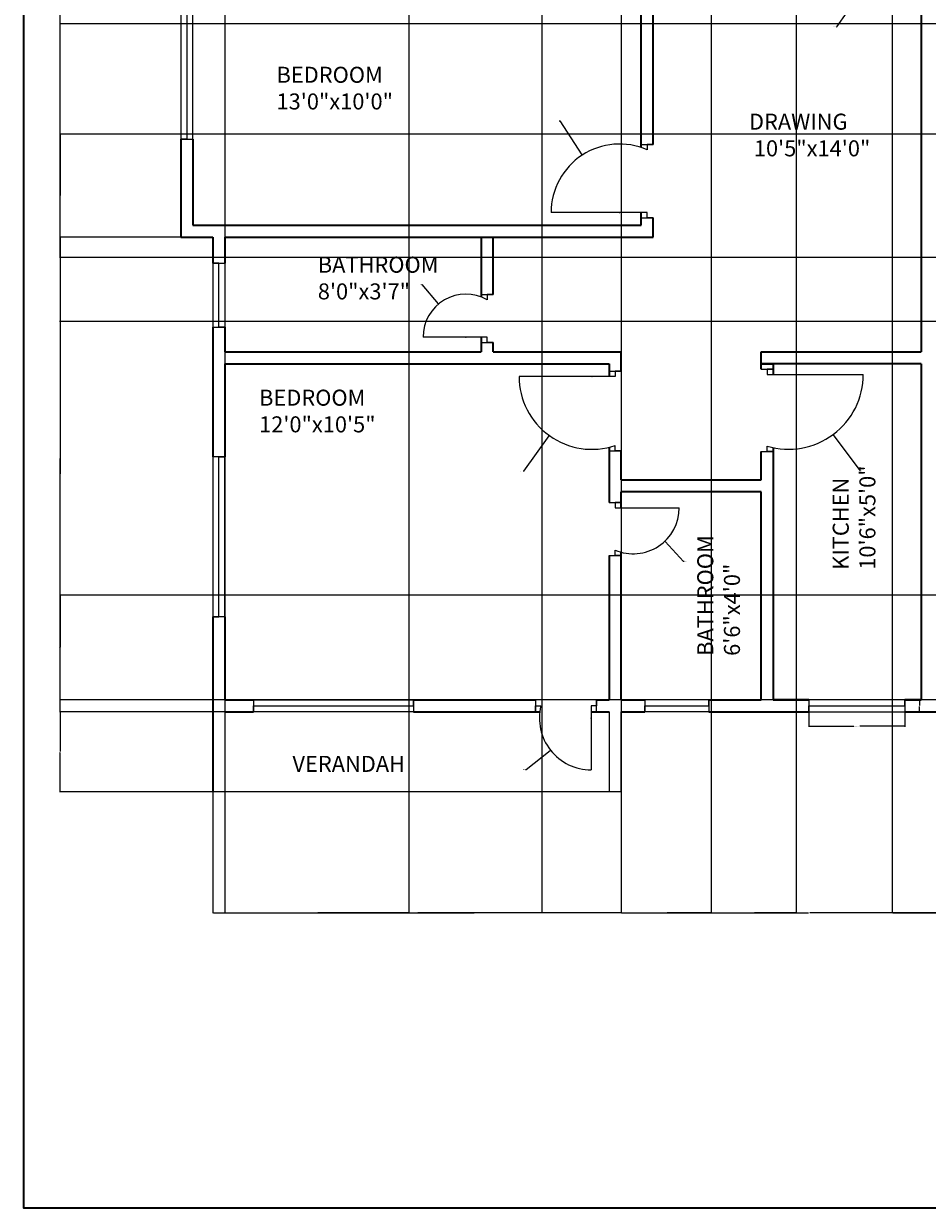
# Model space of a CAD drawing. Units: inches. Extents: x 1831 to 2867, y 1605 to 2524.
# Tile 1 of 7: x 1831 to 2170, y 1605 to 2049. Entities that reach past the tile are written whole.
import ezdxf

# ---------------------------------------------------------------- set-up
doc = ezdxf.new("R2010")
doc.units = ezdxf.units.IN
for name, color, linetype, lineweight in [('A-ANNO-DIMS', 2, 'Continuous', 18), ('A-ANNO-TTLB', 7, 'Continuous', 35), ('A-AREA-IDEN', 7, 'Continuous', 18), ('A-DOOR', 11, 'Continuous', 18), ('A-FLOR-BALC', 7, 'Continuous', 25), ('A-GLAZ', 121, 'Continuous', 18), ('A-WALL', 7, 'Continuous', 35)]:
    doc.layers.add(name, color=color, linetype=linetype, lineweight=lineweight)
doc.styles.get("Standard").update_dxf_attribs({"font": 'arial.ttf'})
doc.dimstyles.get("Standard").update_dxf_attribs({"dimtxt": 0.18, "dimasz": 0.18, "dimexe": 0.18, "dimexo": 0.0625, "dimgap": 0.09, "dimtad": 0, "dimtih": 1, "dimtoh": 1, "dimdec": 4, "dimzin": 0, "dimdsep": 46, "dimtxsty": 'Standard', "dimcen": 0.09, "dimadec": 0, "dimazin": 0, "dimtfac": 1, "dimtdec": 4, "dimtofl": 0, "dimtmove": 0, "dimatfit": 3, "dimfxl": 1, "dimtolj": 1, "dimtzin": 0, "dimarcsym": 0})

# ---------------------------------------------------------------- blocks, each defined once
blk = doc.blocks.new('WIN-60IN')
for p, q in [((4.5, 60), (0, 60)), ((0, 60), (2.25, 60)), ((0, 0), (0, 60)), ((2.25, 60), (2.25, 0)), ((4.5, 60), (4.5, 0)), ((4.5, 0), (0, 0)), ((2.25, 0), (4.5, 0))]:
    blk.add_line(p, q)
blk = doc.blocks.new('WIN-24IN')
for p, q in [((4.5, 24), (0, 24)), ((0, 24), (2.25, 24)), ((0, 0), (0, 24)), ((2.25, 24), (2.25, 0)), ((4.5, 0), (4.5, 24)), ((4.5, 0), (0, 0)), ((2.25, 0), (4.5, 0))]:
    blk.add_line(p, q)
blk = doc.blocks.new('WIN-36IN')
for p, q in [((0, 0), (0, 4.5)), ((36, 4.5), (0, 4.5)), ((36, 0), (36, 4.5)), ((36, 4.5), (36, 2.25)), ((36, 2.25), (0, 2.25)), ((0, 2.25), (0, 0)), ((0, 0), (36, 0))]:
    blk.add_line(p, q)
blk = doc.blocks.new('DOOR-LEAF-36IN')
for p, q in [((0, 2), (4.5, 2)), ((4.5, 2), (2.25, 2)), ((2.25, 2), (2.25, 0)), ((2.25, 0), (38.25, 0))]:
    blk.add_line(p, q)
blk = doc.blocks.new('DOOR-LEAF-36IN-ALT')
for p, q in [((36, 2), (0, 2)), ((33.75, 0), (38.25, 0)), ((36, 0), (36, 2)), ((38.25, 0), (36, 0))]:
    blk.add_line(p, q)
blk = doc.blocks.new('DOOR-LEAF-24IN')
for p, q in [((2.25, 0), (2.25, 2)), ((2.25, 2), (26.25, 2)), ((0, 0), (4.5, 0)), ((4.5, 0), (2.25, 0))]:
    blk.add_line(p, q)
blk = doc.blocks.new('DOOR-LEAF-24IN-ALT')
for p, q in [((24, 2), (0, 2)), ((21.75, 0), (26.25, 0)), ((24, 0), (24, 2)), ((26.25, 0), (24, 0))]:
    blk.add_line(p, q)
blk = doc.blocks.new('DOOR-STRIKE-JAMB')
for p, q in [((0, 0), (4.5, 0)), ((2.25, 0), (2.25, 2)), ((4.5, 0), (2.25, 0))]:
    blk.add_line(p, q)
blk = doc.blocks.new('*D18')
at = {"layer": 'A-ANNO-DIMS', "color": 0, "lineweight": -2, "transparency": 16777216}
for p, q in [((2125.43, 1791.11), (2125.43, 1785.59)), ((2161.43, 1791.11), (2161.43, 1785.59)), ((2125.61, 1785.77), (2142.31, 1785.77)), ((2161.25, 1785.77), (2144.55, 1785.77))]:
    blk.add_line(p, q, dxfattribs=at)
at = {"layer": 'A-ANNO-DIMS', "color": 0, "transparency": 16777216}
for points in [[(2125.61, 1785.8), (2125.61, 1785.74), (2125.43, 1785.77)], [(2161.25, 1785.8), (2161.25, 1785.74), (2161.43, 1785.77)]]:
    blk.add_solid(points, dxfattribs=at)
at = {"layer": 'Defpoints', "color": 0, "transparency": 16777216}
for p in [(2125.43, 1791.17), (2161.43, 1791.17), (2125.43, 1785.77)]:
    blk.add_point(p, dxfattribs=at)
at = {"layer": 'A-ANNO-DIMS', "color": 0, "transparency": 16777216, "insert": (2143.43, 1785.77), "char_height": 0.18, "attachment_point": 5}
blk.add_mtext('\\A1;WINDOW 36 TYP.', dxfattribs=at)
blk = doc.blocks.new('*D19')
at = {"layer": 'A-ANNO-DIMS', "color": 0, "lineweight": -2, "transparency": 16777216}
for p, q in [((2161.49, 1795.67), (2167.01, 1795.67)), ((2166.83, 1795.49), (2166.83, 1793.61)), ((2161.49, 1791.17), (2167.01, 1791.17)), ((2166.83, 1791.35), (2166.83, 1793.24))]:
    blk.add_line(p, q, dxfattribs=at)
at = {"layer": 'A-ANNO-DIMS', "color": 0, "transparency": 16777216}
for points in [[(2166.8, 1795.49), (2166.86, 1795.49), (2166.83, 1795.67)], [(2166.8, 1791.35), (2166.86, 1791.35), (2166.83, 1791.17)]]:
    blk.add_solid(points, dxfattribs=at)
at = {"layer": 'Defpoints', "color": 0, "transparency": 16777216}
for p in [(2161.43, 1795.67), (2161.43, 1791.17), (2166.83, 1791.17)]:
    blk.add_point(p, dxfattribs=at)
at = {"layer": 'A-ANNO-DIMS', "color": 0, "transparency": 16777216, "insert": (2166.83, 1793.42), "char_height": 0.18, "attachment_point": 5}
blk.add_mtext('\\A1;5 TYP.', dxfattribs=at)
blk = doc.blocks.new('*D24')
at = {"layer": 'A-ANNO-DIMS', "color": 0, "lineweight": -2, "transparency": 16777216}
for p, q in [((1902.05, 1761.11), (1902.05, 1715.69)), ((2055.05, 1761.11), (2055.05, 1715.69)), ((1902.23, 1715.87), (1978.27, 1715.87)), ((2054.87, 1715.87), (1978.83, 1715.87))]:
    blk.add_line(p, q, dxfattribs=at)
at = {"layer": 'A-ANNO-DIMS', "color": 0, "transparency": 16777216}
for points in [[(1902.23, 1715.9), (1902.23, 1715.84), (1902.05, 1715.87)], [(2054.87, 1715.9), (2054.87, 1715.84), (2055.05, 1715.87)]]:
    blk.add_solid(points, dxfattribs=at)
at = {"layer": 'Defpoints', "color": 0, "transparency": 16777216}
for p in [(1902.05, 1761.17), (2055.05, 1761.17), (2055.05, 1715.87)]:
    blk.add_point(p, dxfattribs=at)
at = {"layer": 'A-ANNO-DIMS', "color": 0, "transparency": 16777216, "insert": (1978.55, 1715.87), "char_height": 0.18, "attachment_point": 5}
blk.add_mtext('\\A1;153', dxfattribs=at)
blk = doc.blocks.new('*D25')
at = {"layer": 'A-ANNO-DIMS', "color": 0, "lineweight": -2, "transparency": 16777216}
for p, q in [((2055.05, 1761.11), (2055.05, 1715.69)), ((2196.05, 1761.11), (2196.05, 1715.69)), ((2055.23, 1715.87), (2125.29, 1715.87)), ((2195.87, 1715.87), (2125.81, 1715.87))]:
    blk.add_line(p, q, dxfattribs=at)
at = {"layer": 'A-ANNO-DIMS', "color": 0, "transparency": 16777216}
for points in [[(2055.23, 1715.9), (2055.23, 1715.84), (2055.05, 1715.87)], [(2195.87, 1715.9), (2195.87, 1715.84), (2196.05, 1715.87)]]:
    blk.add_solid(points, dxfattribs=at)
at = {"layer": 'Defpoints', "color": 0, "transparency": 16777216}
for p in [(2055.05, 1761.17), (2196.05, 1761.17), (2196.05, 1715.87)]:
    blk.add_point(p, dxfattribs=at)
at = {"layer": 'A-ANNO-DIMS', "color": 0, "transparency": 16777216, "insert": (2125.55, 1715.87), "char_height": 0.18, "attachment_point": 5}
blk.add_mtext('\\A1;141', dxfattribs=at)
blk = doc.blocks.new('*D33')
at = {"layer": 'A-ANNO-DIMS', "color": 0, "lineweight": -2, "transparency": 16777216}
for p, q in [((1889.99, 2218.17), (1844.57, 2218.17)), ((1844.75, 2217.99), (1844.75, 2093.86)), ((1844.75, 1969.35), (1844.75, 2093.49)), ((1889.99, 1969.17), (1844.57, 1969.17))]:
    blk.add_line(p, q, dxfattribs=at)
at = {"layer": 'A-ANNO-DIMS', "color": 0, "transparency": 16777216}
for points in [[(1844.72, 2217.99), (1844.78, 2217.99), (1844.75, 2218.17)], [(1844.72, 1969.35), (1844.78, 1969.35), (1844.75, 1969.17)]]:
    blk.add_solid(points, dxfattribs=at)
at = {"layer": 'Defpoints', "color": 0, "transparency": 16777216}
for p in [(1890.05, 2218.17), (1844.75, 1969.17), (1890.05, 1969.17)]:
    blk.add_point(p, dxfattribs=at)
at = {"layer": 'A-ANNO-DIMS', "color": 0, "transparency": 16777216, "insert": (1844.75, 2093.67), "char_height": 0.18, "attachment_point": 5}
blk.add_mtext('\\A1;249', dxfattribs=at)
blk = doc.blocks.new('*D34')
at = {"layer": 'A-ANNO-DIMS', "color": 0, "lineweight": -2, "transparency": 16777216}
for p, q in [((1901.99, 1969.17), (1844.57, 1969.17)), ((1844.75, 1968.99), (1844.75, 1880.36)), ((1844.75, 1791.35), (1844.75, 1879.99)), ((1906.49, 1791.17), (1844.57, 1791.17))]:
    blk.add_line(p, q, dxfattribs=at)
at = {"layer": 'A-ANNO-DIMS', "color": 0, "transparency": 16777216}
for points in [[(1844.72, 1968.99), (1844.78, 1968.99), (1844.75, 1969.17)], [(1844.72, 1791.35), (1844.78, 1791.35), (1844.75, 1791.17)]]:
    blk.add_solid(points, dxfattribs=at)
at = {"layer": 'Defpoints', "color": 0, "transparency": 16777216}
for p in [(1902.05, 1969.17), (1844.75, 1791.17), (1906.55, 1791.17)]:
    blk.add_point(p, dxfattribs=at)
at = {"layer": 'A-ANNO-DIMS', "color": 0, "transparency": 16777216, "insert": (1844.75, 1880.17), "char_height": 0.18, "attachment_point": 5}
blk.add_mtext('\\A1;178', dxfattribs=at)
blk = doc.blocks.new('*D35')
at = {"layer": 'A-ANNO-DIMS', "color": 0, "lineweight": -2, "transparency": 16777216}
for p, q in [((1906.49, 1791.17), (1844.57, 1791.17)), ((1844.75, 1790.99), (1844.75, 1776.36)), ((1844.75, 1761.35), (1844.75, 1775.99)), ((1901.99, 1761.17), (1844.57, 1761.17))]:
    blk.add_line(p, q, dxfattribs=at)
at = {"layer": 'A-ANNO-DIMS', "color": 0, "transparency": 16777216}
for points in [[(1844.72, 1790.99), (1844.78, 1790.99), (1844.75, 1791.17)], [(1844.72, 1761.35), (1844.78, 1761.35), (1844.75, 1761.17)]]:
    blk.add_solid(points, dxfattribs=at)
at = {"layer": 'Defpoints', "color": 0, "transparency": 16777216}
for p in [(1906.55, 1791.17), (1844.75, 1761.17), (1902.05, 1761.17)]:
    blk.add_point(p, dxfattribs=at)
at = {"layer": 'A-ANNO-DIMS', "color": 0, "transparency": 16777216, "insert": (1844.75, 1776.17), "char_height": 0.18, "attachment_point": 5}
blk.add_mtext('\\A1;30', dxfattribs=at)
blk = doc.blocks.new('*D37')
at = {"layer": 'A-ANNO-DIMS', "color": 0, "lineweight": -2, "transparency": 16777216}
for p, q in [((1906.55, 2387.11), (1906.55, 1715.69)), ((1975.47, 2387.11), (1975.47, 1715.69)), ((1906.73, 1715.87), (1940.62, 1715.87)), ((1975.29, 1715.87), (1941.4, 1715.87))]:
    blk.add_line(p, q, dxfattribs=at)
at = {"layer": 'A-ANNO-DIMS', "color": 0, "transparency": 16777216}
for points in [[(1906.73, 1715.9), (1906.73, 1715.84), (1906.55, 1715.87)], [(1975.29, 1715.9), (1975.29, 1715.84), (1975.47, 1715.87)]]:
    blk.add_solid(points, dxfattribs=at)
at = {"layer": 'Defpoints', "color": 0, "transparency": 16777216}
for p in [(1906.55, 2387.17), (1975.47, 2387.17), (1975.47, 1715.87)]:
    blk.add_point(p, dxfattribs=at)
at = {"layer": 'A-ANNO-DIMS', "color": 0, "transparency": 16777216, "insert": (1941.01, 1715.87), "char_height": 0.18, "attachment_point": 5}
blk.add_mtext('\\A1;68.92', dxfattribs=at)
blk = doc.blocks.new('*D38')
at = {"layer": 'A-ANNO-DIMS', "color": 0, "lineweight": -2, "transparency": 16777216}
for p, q in [((1975.47, 2391.61), (1975.47, 1715.69)), ((2025.28, 2391.61), (2025.28, 1715.69)), ((1975.65, 1715.87), (1999.99, 1715.87)), ((2025.1, 1715.87), (2000.75, 1715.87))]:
    blk.add_line(p, q, dxfattribs=at)
at = {"layer": 'A-ANNO-DIMS', "color": 0, "transparency": 16777216}
for points in [[(1975.65, 1715.9), (1975.65, 1715.84), (1975.47, 1715.87)], [(2025.1, 1715.9), (2025.1, 1715.84), (2025.28, 1715.87)]]:
    blk.add_solid(points, dxfattribs=at)
at = {"layer": 'Defpoints', "color": 0, "transparency": 16777216}
for p in [(1975.47, 2391.67), (2025.28, 2391.67), (2025.28, 1715.87)]:
    blk.add_point(p, dxfattribs=at)
at = {"layer": 'A-ANNO-DIMS', "color": 0, "transparency": 16777216, "insert": (2000.37, 1715.87), "char_height": 0.18, "attachment_point": 5}
blk.add_mtext('\\A1;49.81', dxfattribs=at)
blk = doc.blocks.new('*D39')
at = {"layer": 'A-ANNO-DIMS', "color": 0, "lineweight": -2, "transparency": 16777216}
for p, q in [((2055.05, 2387.11), (2055.05, 1715.69)), ((2088.73, 2387.11), (2088.73, 1715.69)), ((2055.23, 1715.87), (2071.5, 1715.87)), ((2088.55, 1715.87), (2072.28, 1715.87))]:
    blk.add_line(p, q, dxfattribs=at)
at = {"layer": 'A-ANNO-DIMS', "color": 0, "transparency": 16777216}
for points in [[(2055.23, 1715.9), (2055.23, 1715.84), (2055.05, 1715.87)], [(2088.55, 1715.9), (2088.55, 1715.84), (2088.73, 1715.87)]]:
    blk.add_solid(points, dxfattribs=at)
at = {"layer": 'Defpoints', "color": 0, "transparency": 16777216}
for p in [(2055.05, 2387.17), (2088.73, 2387.17), (2088.73, 1715.87)]:
    blk.add_point(p, dxfattribs=at)
at = {"layer": 'A-ANNO-DIMS', "color": 0, "transparency": 16777216, "insert": (2071.89, 1715.87), "char_height": 0.18, "attachment_point": 5}
blk.add_mtext('\\A1;33.68', dxfattribs=at)
blk = doc.blocks.new('*D40')
at = {"layer": 'A-ANNO-DIMS', "color": 0, "lineweight": -2, "transparency": 16777216}
for p, q in [((2088.73, 2387.11), (2088.73, 1715.69)), ((2120.64, 2387.11), (2120.64, 1715.69)), ((2088.91, 1715.87), (2104.31, 1715.87)), ((2120.46, 1715.87), (2105.06, 1715.87))]:
    blk.add_line(p, q, dxfattribs=at)
at = {"layer": 'A-ANNO-DIMS', "color": 0, "transparency": 16777216}
for points in [[(2088.91, 1715.9), (2088.91, 1715.84), (2088.73, 1715.87)], [(2120.46, 1715.9), (2120.46, 1715.84), (2120.64, 1715.87)]]:
    blk.add_solid(points, dxfattribs=at)
at = {"layer": 'Defpoints', "color": 0, "transparency": 16777216}
for p in [(2088.73, 2387.17), (2120.64, 2387.17), (2120.64, 1715.87)]:
    blk.add_point(p, dxfattribs=at)
at = {"layer": 'A-ANNO-DIMS', "color": 0, "transparency": 16777216, "insert": (2104.69, 1715.87), "char_height": 0.18, "attachment_point": 5}
blk.add_mtext('\\A1;31.91', dxfattribs=at)
blk = doc.blocks.new('*D41')
at = {"layer": 'A-ANNO-DIMS', "color": 0, "lineweight": -2, "transparency": 16777216}
for p, q in [((2156.64, 2387.11), (2156.64, 1715.69)), ((2210.17, 2387.11), (2210.17, 1715.69)), ((2156.82, 1715.87), (2183.01, 1715.87)), ((2209.99, 1715.87), (2183.8, 1715.87))]:
    blk.add_line(p, q, dxfattribs=at)
at = {"layer": 'A-ANNO-DIMS', "color": 0, "transparency": 16777216}
for points in [[(2156.82, 1715.9), (2156.82, 1715.84), (2156.64, 1715.87)], [(2209.99, 1715.9), (2209.99, 1715.84), (2210.17, 1715.87)]]:
    blk.add_solid(points, dxfattribs=at)
at = {"layer": 'Defpoints', "color": 0, "transparency": 16777216}
for p in [(2156.64, 2387.17), (2210.17, 2387.17), (2210.17, 1715.87)]:
    blk.add_point(p, dxfattribs=at)
at = {"layer": 'A-ANNO-DIMS', "color": 0, "transparency": 16777216, "insert": (2183.4, 1715.87), "char_height": 0.18, "attachment_point": 5}
blk.add_mtext('\\A1;53.52', dxfattribs=at)
blk = doc.blocks.new('*D53')
at = {"layer": 'A-ANNO-DIMS', "color": 0, "lineweight": -2, "transparency": 16777216}
for p, q in [((2786.99, 2007.7), (1844.57, 2007.7)), ((1844.75, 2007.52), (1844.75, 1984.78)), ((1844.75, 1961.67), (1844.75, 1984.41)), ((2786.99, 1961.49), (1844.57, 1961.49))]:
    blk.add_line(p, q, dxfattribs=at)
at = {"layer": 'A-ANNO-DIMS', "color": 0, "transparency": 16777216}
for points in [[(1844.72, 2007.52), (1844.78, 2007.52), (1844.75, 2007.7)], [(1844.72, 1961.67), (1844.78, 1961.67), (1844.75, 1961.49)]]:
    blk.add_solid(points, dxfattribs=at)
at = {"layer": 'Defpoints', "color": 0, "transparency": 16777216}
for p in [(2787.05, 2007.7), (1844.75, 1961.49), (2787.05, 1961.49)]:
    blk.add_point(p, dxfattribs=at)
at = {"layer": 'A-ANNO-DIMS', "color": 0, "transparency": 16777216, "insert": (1844.75, 1984.59), "char_height": 0.18, "attachment_point": 5}
blk.add_mtext('\\A1;46.2', dxfattribs=at)
blk = doc.blocks.new('*D54')
at = {"layer": 'A-ANNO-DIMS', "color": 0, "lineweight": -2, "transparency": 16777216}
for p, q in [((2786.99, 1937.49), (1844.57, 1937.49)), ((1844.75, 1937.31), (1844.75, 1886.37)), ((1844.75, 1835.06), (1844.75, 1886)), ((2786.99, 1834.88), (1844.57, 1834.88))]:
    blk.add_line(p, q, dxfattribs=at)
at = {"layer": 'A-ANNO-DIMS', "color": 0, "transparency": 16777216}
for points in [[(1844.72, 1937.31), (1844.78, 1937.31), (1844.75, 1937.49)], [(1844.72, 1835.06), (1844.78, 1835.06), (1844.75, 1834.88)]]:
    blk.add_solid(points, dxfattribs=at)
at = {"layer": 'Defpoints', "color": 0, "transparency": 16777216}
for p in [(2787.05, 1937.49), (1844.75, 1834.88), (2787.05, 1834.88)]:
    blk.add_point(p, dxfattribs=at)
at = {"layer": 'A-ANNO-DIMS', "color": 0, "transparency": 16777216, "insert": (1844.75, 1886.19), "char_height": 0.18, "attachment_point": 5}
blk.add_mtext('\\A1;102.61', dxfattribs=at)
blk = doc.blocks.new('*D55')
at = {"layer": 'A-ANNO-DIMS', "color": 0, "lineweight": -2, "transparency": 16777216}
for p, q in [((2786.99, 1834.88), (1844.57, 1834.88)), ((1844.75, 1834.7), (1844.75, 1815.46)), ((1844.75, 1795.85), (1844.75, 1815.09)), ((2786.99, 1795.67), (1844.57, 1795.67))]:
    blk.add_line(p, q, dxfattribs=at)
at = {"layer": 'A-ANNO-DIMS', "color": 0, "transparency": 16777216}
for points in [[(1844.72, 1834.7), (1844.78, 1834.7), (1844.75, 1834.88)], [(1844.72, 1795.85), (1844.78, 1795.85), (1844.75, 1795.67)]]:
    blk.add_solid(points, dxfattribs=at)
at = {"layer": 'Defpoints', "color": 0, "transparency": 16777216}
for p in [(2787.05, 1834.88), (1844.75, 1795.67), (2787.05, 1795.67)]:
    blk.add_point(p, dxfattribs=at)
at = {"layer": 'A-ANNO-DIMS', "color": 0, "transparency": 16777216, "insert": (1844.75, 1815.28), "char_height": 0.18, "attachment_point": 5}
blk.add_mtext('\\A1;39.206', dxfattribs=at)
blk = doc.blocks.new('*D60')
at = {"layer": 'A-ANNO-DIMS', "color": 0, "lineweight": -2, "transparency": 16777216}
for p, q in [((2225.43, 2091.42), (1844.57, 2091.42)), ((1844.75, 2091.24), (1844.75, 2070.48)), ((1844.75, 2049.35), (1844.75, 2070.12)), ((2225.43, 2049.17), (1844.57, 2049.17))]:
    blk.add_line(p, q, dxfattribs=at)
at = {"layer": 'A-ANNO-DIMS', "color": 0, "transparency": 16777216}
for points in [[(1844.72, 2091.24), (1844.78, 2091.24), (1844.75, 2091.42)], [(1844.72, 2049.35), (1844.78, 2049.35), (1844.75, 2049.17)]]:
    blk.add_solid(points, dxfattribs=at)
at = {"layer": 'Defpoints', "color": 0, "transparency": 16777216}
for p in [(1844.75, 2091.42), (2225.49, 2091.42), (2225.49, 2049.17)]:
    blk.add_point(p, dxfattribs=at)
at = {"layer": 'A-ANNO-DIMS', "color": 0, "transparency": 16777216, "insert": (1844.75, 2070.3), "char_height": 0.18, "attachment_point": 5}
blk.add_mtext('\\A1;42.25', dxfattribs=at)
blk = doc.blocks.new('*D73')
at = {"layer": 'A-ANNO-DIMS', "color": 0, "lineweight": -2, "transparency": 16777216}
for p, q in [((2117.68, 1917.66), (2117.86, 1917.66)), ((2117.77, 1917.57), (2117.77, 1917.75)), ((2144.6, 1881.73), (2134.65, 1895.06)), ((2144.78, 1881.73), (2144.6, 1881.73))]:
    blk.add_line(p, q, dxfattribs=at)
at = {"layer": 'A-ANNO-DIMS', "color": 0, "transparency": 16777216}
blk.add_solid([(2134.67, 1895.08), (2134.62, 1895.04), (2134.54, 1895.2)], dxfattribs=at)
at = {"layer": 'Defpoints', "color": 0, "transparency": 16777216}
for p in [(2117.77, 1917.66), (2134.54, 1895.2)]:
    blk.add_point(p, dxfattribs=at)
at = {"layer": 'A-ANNO-DIMS', "color": 0, "transparency": 16777216, "insert": (2145.26, 1881.73), "char_height": 0.18, "attachment_point": 5}
blk.add_mtext('\\A1;R28.03', dxfattribs=at)
blk = doc.blocks.new('*D77')
at = {"layer": 'A-ANNO-DIMS', "color": 0, "lineweight": -2, "transparency": 16777216}
for p, q in [((2044.03, 1916.93), (2044.21, 1916.93)), ((2044.12, 1916.84), (2044.12, 1917.02)), ((2018.59, 1881.45), (2028.06, 1894.61)), ((2018.41, 1881.45), (2018.59, 1881.45))]:
    blk.add_line(p, q, dxfattribs=at)
at = {"layer": 'A-ANNO-DIMS', "color": 0, "transparency": 16777216}
blk.add_solid([(2028.04, 1894.63), (2028.08, 1894.59), (2028.17, 1894.76)], dxfattribs=at)
at = {"layer": 'Defpoints', "color": 0, "transparency": 16777216}
for p in [(2044.12, 1916.93), (2028.17, 1894.76)]:
    blk.add_point(p, dxfattribs=at)
at = {"layer": 'A-ANNO-DIMS', "color": 0, "transparency": 16777216, "insert": (2017.86, 1881.45), "char_height": 0.18, "attachment_point": 5}
blk.add_mtext('\\A1;R27.315', dxfattribs=at)
blk = doc.blocks.new('*D79')
at = {"layer": 'A-ANNO-DIMS', "color": 0, "lineweight": -2, "transparency": 16777216}
for p, q in [((2160.66, 2083.26), (2160.84, 2083.26)), ((2160.75, 2083.17), (2160.75, 2083.35)), ((2135.91, 2048.03), (2145.12, 2061.09)), ((2135.73, 2048.03), (2135.91, 2048.03))]:
    blk.add_line(p, q, dxfattribs=at)
at = {"layer": 'A-ANNO-DIMS', "color": 0, "transparency": 16777216}
blk.add_solid([(2145.09, 2061.11), (2145.14, 2061.08), (2145.22, 2061.24)], dxfattribs=at)
at = {"layer": 'Defpoints', "color": 0, "transparency": 16777216}
for p in [(2160.75, 2083.26), (2145.22, 2061.24)]:
    blk.add_point(p, dxfattribs=at)
at = {"layer": 'A-ANNO-DIMS', "color": 0, "transparency": 16777216, "insert": (2135.18, 2048.03), "char_height": 0.18, "attachment_point": 5}
blk.add_mtext('\\A1;R26.945', dxfattribs=at)
blk = doc.blocks.new('*D83')
at = {"layer": 'A-ANNO-DIMS', "color": 0, "lineweight": -2, "transparency": 16777216}
for p, q in [((2031.86, 2012.78), (2032.04, 2012.78)), ((2032.04, 2012.78), (2040.34, 2000.04)), ((2054.36, 1978.4), (2054.54, 1978.4)), ((2054.45, 1978.31), (2054.45, 1978.49))]:
    blk.add_line(p, q, dxfattribs=at)
at = {"layer": 'A-ANNO-DIMS', "color": 0, "transparency": 16777216}
blk.add_solid([(2040.37, 2000.05), (2040.32, 2000.02), (2040.44, 1999.89)], dxfattribs=at)
at = {"layer": 'Defpoints', "color": 0, "transparency": 16777216}
for p in [(2040.44, 1999.89), (2054.45, 1978.4)]:
    blk.add_point(p, dxfattribs=at)
at = {"layer": 'A-ANNO-DIMS', "color": 0, "transparency": 16777216, "insert": (2031.38, 2012.78), "char_height": 0.18, "attachment_point": 5}
blk.add_mtext('\\A1;R25.65', dxfattribs=at)
blk = doc.blocks.new('*D87')
at = {"layer": 'A-ANNO-DIMS', "color": 0, "lineweight": -2, "transparency": 16777216}
for p, q in [((2043.75, 1788.85), (2043.93, 1788.85)), ((2043.84, 1788.76), (2043.84, 1788.94)), ((2019.41, 1769.63), (2028.43, 1776.73)), ((2019.23, 1769.63), (2019.41, 1769.63))]:
    blk.add_line(p, q, dxfattribs=at)
at = {"layer": 'A-ANNO-DIMS', "color": 0, "transparency": 16777216}
blk.add_solid([(2028.41, 1776.75), (2028.45, 1776.7), (2028.57, 1776.84)], dxfattribs=at)
at = {"layer": 'Defpoints', "color": 0, "transparency": 16777216}
for p in [(2043.84, 1788.85), (2028.57, 1776.84)]:
    blk.add_point(p, dxfattribs=at)
at = {"layer": 'A-ANNO-DIMS', "color": 0, "transparency": 16777216, "insert": (2018.68, 1769.63), "char_height": 0.18, "attachment_point": 5}
blk.add_mtext('\\A1;R19.428', dxfattribs=at)
blk = doc.blocks.new('*D96')
at = {"layer": 'A-ANNO-DIMS', "color": 0, "lineweight": -2, "transparency": 16777216}
for p, q in [((1980.19, 1951.42), (1980.37, 1951.42)), ((1980.37, 1951.42), (1986.44, 1944.17)), ((1996.77, 1931.71), (1996.95, 1931.71)), ((1996.86, 1931.62), (1996.86, 1931.8))]:
    blk.add_line(p, q, dxfattribs=at)
at = {"layer": 'A-ANNO-DIMS', "color": 0, "transparency": 16777216}
blk.add_solid([(1986.46, 1944.19), (1986.42, 1944.15), (1986.56, 1944.03)], dxfattribs=at)
at = {"layer": 'Defpoints', "color": 0, "transparency": 16777216}
for p in [(1986.56, 1944.03), (1996.86, 1931.71)]:
    blk.add_point(p, dxfattribs=at)
at = {"layer": 'A-ANNO-DIMS', "color": 0, "transparency": 16777216, "insert": (1979.71, 1951.42), "char_height": 0.18, "attachment_point": 5}
blk.add_mtext('\\A1;R16.06', dxfattribs=at)
blk = doc.blocks.new('*D97')
at = {"layer": 'A-ANNO-DIMS', "color": 0, "lineweight": -2, "transparency": 16777216}
for p, q in [((2059.48, 1867.69), (2059.66, 1867.69)), ((2059.57, 1867.6), (2059.57, 1867.78)), ((2078.45, 1847.6), (2071.5, 1855)), ((2078.63, 1847.6), (2078.45, 1847.6))]:
    blk.add_line(p, q, dxfattribs=at)
at = {"layer": 'A-ANNO-DIMS', "color": 0, "transparency": 16777216}
blk.add_solid([(2071.52, 1855.02), (2071.47, 1854.98), (2071.37, 1855.14)], dxfattribs=at)
at = {"layer": 'Defpoints', "color": 0, "transparency": 16777216}
for p in [(2059.57, 1867.69), (2071.37, 1855.14)]:
    blk.add_point(p, dxfattribs=at)
at = {"layer": 'A-ANNO-DIMS', "color": 0, "transparency": 16777216, "insert": (2079.11, 1847.6), "char_height": 0.18, "attachment_point": 5}
blk.add_mtext('\\A1;R17.23', dxfattribs=at)

msp = doc.modelspace()

# ---------------------------------------------------------------- linework, layer by layer
at = {"layer": 'A-ANNO-TTLB'}
msp.add_lwpolyline([(1831.1248, 2523.9204), (2867.0416, 2523.9204), (2867.0416, 1605.0781), (1831.1248, 1605.0781)], close=True, dxfattribs=at)
at = {"layer": 'A-DOOR'}
for centre, radius, start, end in [((2054.453, 1978.3983), 25.6519, 66.208959, 180), ((1996.8625, 1931.7112), 16.0615, 60.379406, 180), ((2044.1157, 1916.9308), 27.3147, 180, 288.540393), ((2117.7728, 1917.6648), 28.0282, 253.475877, 360), ((2059.5721, 1867.688), 17.2289, 246.858029, 360), ((2043.8406, 1788.8513), 19.4276, 166.38723, 270)]:
    msp.add_arc(centre, radius, start, end, dxfattribs=at)
at = {"layer": 'A-FLOR-BALC'}
for p, q in [((1906.551, 1791.1738), (1906.551, 1761.1738)), ((2050.551, 1791.1738), (2050.551, 1761.1738)), ((2055.051, 1761.1738), (2055.051, 1791.1738)), ((2055.051, 1761.1738), (1902.051, 1761.1738))]:
    msp.add_line(p, q, dxfattribs=at)
at = {"layer": 'A-WALL'}
for p, q in [((2062.551, 2002.7385), (2062.551, 2089.1738)), ((2067.051, 2003.8704), (2067.051, 2089.1738)), ((2167.551, 2057.1926), (2167.551, 1926.1738)), ((1890.051, 2005.8506), (1890.051, 1969.1738)), ((1894.551, 2005.8506), (1894.551, 1973.6738)), ((2062.551, 1973.6738), (2062.551, 1978.3983)), ((2067.051, 1969.1738), (2067.051, 1976.3983)), ((1894.551, 1973.6738), (2062.551, 1973.6738)), ((1890.051, 1969.1738), (1902.051, 1969.1738)), ((1902.051, 1969.1738), (1902.051, 1959.4423)), ((1906.551, 1969.1738), (1906.551, 1959.4423)), ((1906.551, 1969.1738), (2067.051, 1969.1738)), ((1906.551, 1969.1738), (2002.551, 1969.1738)), ((2002.551, 1969.1738), (2002.551, 1946.7317)), ((2007.051, 1947.6738), (2007.051, 1969.1738)), ((1902.051, 1935.4423), (1902.051, 1886.7859)), ((1906.551, 1935.4423), (1906.551, 1926.1738)), ((2002.551, 1931.7112), (2002.551, 1926.1738)), ((2007.051, 1926.1738), (2007.051, 1929.7112)), ((1906.551, 1926.1738), (2002.551, 1926.1738)), ((2007.051, 1926.1738), (2055.051, 1926.1738)), ((2055.051, 1918.9308), (2055.051, 1926.1738)), ((2107.551, 1926.1738), (2167.551, 1926.1738)), ((2107.551, 1919.6648), (2107.551, 1926.1738)), ((1906.551, 1921.6738), (2050.551, 1921.6738)), ((1906.551, 1921.6738), (2050.551, 1921.6738)), ((1906.551, 1921.6738), (1906.551, 1886.7859)), ((2050.551, 1921.6738), (2050.551, 1916.9308)), ((2167.551, 1921.6738), (2107.551, 1921.6738)), ((2107.551, 1921.6738), (2112.051, 1921.6738)), ((2112.051, 1921.6738), (2112.051, 1917.6648)), ((2167.551, 1921.6738), (2167.551, 1795.6738)), ((2050.551, 1890.385), (2050.551, 1869.688)), ((2055.051, 1878.1738), (2055.051, 1889.0338)), ((2107.551, 1878.1738), (2107.551, 1888.7941)), ((2112.051, 1890.2268), (2112.051, 1795.6738)), ((2055.051, 1878.1738), (2107.551, 1878.1738)), ((2107.551, 1873.6738), (2055.051, 1873.6738)), ((2055.051, 1867.688), (2055.051, 1873.6738)), ((2107.551, 1795.6738), (2107.551, 1873.6738)), ((2107.551, 1795.6738), (2107.551, 1873.6738)), ((2050.551, 1849.8455), (2050.551, 1795.6738)), ((2055.051, 1795.6738), (2055.051, 1851.063)), ((1902.051, 1826.7859), (1902.051, 1761.1738)), ((1906.551, 1826.7859), (1906.551, 1795.6738)), ((1906.551, 1795.6738), (1917.2343, 1795.6738)), ((1977.2343, 1795.6738), (2022.9588, 1795.6738)), ((2045.8406, 1795.6738), (2050.551, 1795.6738)), ((2055.051, 1795.6738), (2063.943, 1795.6738)), ((2087.943, 1795.6738), (2107.551, 1795.6738)), ((2125.4296, 1795.6738), (2112.051, 1795.6738)), ((2112.051, 1795.6738), (2125.4296, 1795.6738)), ((2167.551, 1795.6738), (2161.4296, 1795.6738)), ((2161.4296, 1795.6738), (2167.551, 1795.6738)), ((1906.551, 1791.1738), (1917.2343, 1791.1738)), ((1977.2343, 1791.1738), (2024.5524, 1791.1738)), ((2043.8406, 1791.1738), (2050.551, 1791.1738)), ((2055.051, 1791.1738), (2063.943, 1791.1738)), ((2087.943, 1791.1738), (2125.4296, 1791.1738)), ((2161.4296, 1791.1738), (2196.051, 1791.1738))]:
    msp.add_line(p, q, dxfattribs=at)

# ---------------------------------------------------------------- block references
at = {"layer": 'A-DOOR', "extrusion": (0, 0, -1), "zscale": -1, "rotation": 180}
for name, p in [('DOOR-STRIKE-JAMB', (-2062.551, 2003.8704)), ('DOOR-STRIKE-JAMB', (-2002.551, 1947.6738)), ('DOOR-LEAF-36IN-ALT', (-2016.801, 1918.9308)), ('DOOR-LEAF-24IN', (-2050.551, 1869.688))]:
    msp.add_blockref(name, p, dxfattribs=at)
at = {"layer": 'A-DOOR'}
for name, p in [('DOOR-LEAF-36IN-ALT', (2028.801, 1976.3983)), ('DOOR-LEAF-24IN-ALT', (1980.801, 1929.7112)), ('DOOR-LEAF-36IN', (2107.551, 1917.6648)), ('DOOR-STRIKE-JAMB', (2050.551, 1889.0338)), ('DOOR-STRIKE-JAMB', (2107.551, 1888.7941)), ('DOOR-STRIKE-JAMB', (2050.551, 1849.8455))]:
    msp.add_blockref(name, p, dxfattribs=at)
for name, p, rotation in [('DOOR-STRIKE-JAMB', (2022.9588, 1795.6738), 270.0000000000025), ('DOOR-LEAF-24IN-ALT', (2045.8406, 1769.4238), 90.00000000000003)]:
    msp.add_blockref(name, p, dxfattribs=dict(at, rotation=rotation))
at = {"layer": 'A-GLAZ', "extrusion": (0, 0, -1), "zscale": -1}
msp.add_blockref('WIN-60IN', (-1894.551, 2005.8506), dxfattribs=at)
at = {"layer": 'A-GLAZ'}
for name, p, rotation in [('WIN-24IN', (1906.551, 1959.4423), 180), ('WIN-60IN', (1977.2343, 1791.1738), 89.99999999999925), ('WIN-24IN', (2087.943, 1791.1738), 89.99999999999827), ('WIN-36IN', (2161.4296, 1795.6738), 180)]:
    msp.add_blockref(name, p, dxfattribs=dict(at, rotation=rotation))
at = {"layer": 'A-GLAZ', "extrusion": (0, 0, -1), "zscale": -1, "rotation": 180}
msp.add_blockref('WIN-60IN', (-1902.051, 1886.7859), dxfattribs=at)

# ---------------------------------------------------------------- texts
at = {"layer": 'A-AREA-IDEN', "char_height": 6, "attachment_point": 1}
for s, width, insert in [('BEDROOM\\P13\'0"x10\'0"', 139.23882, (1925.8839, 2033.0244)), ('DRAWING\\P 10\'5"x14\'0"', 177.829253, (2102.963, 2015.4476)), ('BATHROOM\\P8\'0"x3\'7"', 130.202265, (1941.3657, 1961.8148)), ('BEDROOM\\P12\'0"x10\'5"', 206.941198, (1919.3563, 1911.9735)), ('VERANDAH', 121.894867, (1931.8573, 1774.6941))]:
    msp.add_mtext_dynamic_manual_height_columns(s, width=width, gutter_width=12.5, heights=[0], dxfattribs=dict(at, insert=insert))
at = {"layer": 'A-AREA-IDEN', "char_height": 6, "attachment_point": 1, "rotation": 90}
for s, width, insert in [('KITCHEN\\P10\'6"x5\'0"', 151.051789, (2134.3486, 1844.4666)), ('BATHROOM\\P6\'6"x4\'0"', 93.191719, (2083.5899, 1812.1792))]:
    msp.add_mtext_dynamic_manual_height_columns(s, width=width, gutter_width=12.5, heights=[0], dxfattribs=dict(at, insert=insert))

# ---------------------------------------------------------------- dimensions: what is measured, and where the dimension line sits
at = {"layer": 'A-ANNO-DIMS'}
for base, p1, p2, override, picture, middle in [((2025.2753, 1715.8738), (1975.4676, 2391.6738), (2025.2753, 2391.6738), {"dimdec": 2, "dimlfac": 1, "dimrnd": 0, "dimzin": 0, "dimdsep": 46, "dimlunit": 2}, '*D38', (2000.3714, 1715.8738)), ((1975.4676, 1715.8738), (1906.551, 2387.1738), (1975.4676, 2387.1738), {"dimdec": 2, "dimlfac": 1, "dimrnd": 0, "dimzin": 0, "dimdsep": 46, "dimlunit": 2}, '*D37', (1941.0093, 1715.8738)), ((2088.7306, 1715.8738), (2055.051, 2387.1738), (2088.7306, 2387.1738), {"dimdec": 2, "dimlfac": 1, "dimrnd": 0, "dimzin": 0, "dimdsep": 46, "dimlunit": 2}, '*D39', (2071.8908, 1715.8738)), ((2120.6429, 1715.8738), (2088.7306, 2387.1738), (2120.6429, 2387.1738), {"dimdec": 2, "dimlfac": 1, "dimrnd": 0, "dimzin": 0, "dimdsep": 46, "dimlunit": 2}, '*D40', (2104.6867, 1715.8738)), ((2210.1653, 1715.8738), (2156.6429, 2387.1738), (2210.1653, 2387.1738), {"dimdec": 2, "dimlfac": 1, "dimrnd": 0, "dimzin": 0, "dimdsep": 46, "dimlunit": 2}, '*D41', (2183.4041, 1715.8738)), ((2055.051, 1715.8738), (1902.051, 1761.1738), (2055.051, 1761.1738), {"dimdec": 0, "dimlfac": 1, "dimrnd": 0, "dimzin": 0, "dimdsep": 46, "dimlunit": 2}, '*D24', (1978.551, 1715.8738)), ((2196.051, 1715.8738), (2055.051, 1761.1738), (2196.051, 1761.1738), {"dimdec": 0, "dimlfac": 1, "dimrnd": 0, "dimzin": 0, "dimdsep": 46, "dimlunit": 2}, '*D25', (2125.551, 1715.8738))]:
    dim = msp.add_linear_dim(base=base, p1=p1, p2=p2, dimstyle='Standard', override=override, dxfattribs=at)
    dim.commit()
    dim.dimension.update_dxf_attribs({"geometry": picture, "text_midpoint": middle})
for base, p1, p2, override, picture, middle in [((1844.751, 1969.1738), (1890.051, 2218.1738), (1890.051, 1969.1738), {"dimdec": 0, "dimlfac": 1, "dimrnd": 0, "dimzin": 0, "dimdsep": 46, "dimlunit": 2}, '*D33', (1844.751, 2093.6738)), ((1844.751, 2091.4238), (2225.4925, 2049.1738), (2225.4925, 2091.4238), {"dimdec": 2, "dimlfac": 1, "dimrnd": 0, "dimzin": 0, "dimdsep": 46, "dimlunit": 2}, '*D60', (1844.751, 2070.2988)), ((1844.751, 1961.4909), (2787.051, 2007.6955), (2787.051, 1961.4909), {"dimdec": 1, "dimlfac": 1, "dimrnd": 0, "dimzin": 0, "dimdsep": 46, "dimlunit": 2}, '*D53', (1844.751, 1984.5932)), ((1844.751, 1791.1738), (1902.051, 1969.1738), (1906.551, 1791.1738), {"dimdec": 0, "dimlfac": 1, "dimrnd": 0, "dimzin": 0, "dimdsep": 46, "dimlunit": 2}, '*D34', (1844.751, 1880.1738)), ((1844.751, 1834.8797), (2787.051, 1937.4909), (2787.051, 1834.8797), {"dimdec": 2, "dimlfac": 1, "dimrnd": 0, "dimzin": 0, "dimdsep": 46, "dimlunit": 2}, '*D54', (1844.751, 1886.1853)), ((1844.751, 1795.6738), (2787.051, 1834.8797), (2787.051, 1795.6738), {"dimdec": 3, "dimlfac": 1, "dimrnd": 0, "dimzin": 0, "dimdsep": 46, "dimlunit": 2}, '*D55', (1844.751, 1815.2767)), ((1844.751, 1761.1738), (1906.551, 1791.1738), (1902.051, 1761.1738), {"dimdec": 0, "dimlfac": 1, "dimrnd": 0, "dimzin": 0, "dimdsep": 46, "dimlunit": 2}, '*D35', (1844.751, 1776.1738))]:
    dim = msp.add_linear_dim(base=base, p1=p1, p2=p2, angle=90, dimstyle='Standard', override=override, dxfattribs=at)
    dim.commit()
    dim.dimension.update_dxf_attribs({"geometry": picture, "text_midpoint": middle})
for center, mpoint, override, picture, middle in [((2160.7458, 2083.2638), (2145.221, 2061.241), {"dimdec": 3, "dimlfac": 1, "dimrnd": 0, "dimzin": 0, "dimdsep": 46, "dimlunit": 2}, '*D79', (2135.1757, 2048.0274)), ((2054.453, 1978.3983), (2040.4427, 1999.8864), {"dimdec": 2, "dimlfac": 1, "dimrnd": 0, "dimzin": 0, "dimdsep": 46, "dimlunit": 2}, '*D83', (2031.3761, 2012.7792)), ((1996.8625, 1931.7112), (1986.5564, 1944.0302), {"dimdec": 2, "dimlfac": 1, "dimrnd": 0, "dimzin": 0, "dimdsep": 46, "dimlunit": 2}, '*D96', (1979.713, 1951.4216)), ((2044.1157, 1916.9308), (2028.1651, 1894.7572), {"dimdec": 3, "dimlfac": 1, "dimrnd": 0, "dimzin": 0, "dimdsep": 46, "dimlunit": 2}, '*D77', (2017.8643, 1881.453)), ((2117.7728, 1917.6648), (2134.5382, 1895.2037), {"dimdec": 2, "dimlfac": 1, "dimrnd": 0, "dimzin": 0, "dimdsep": 46, "dimlunit": 2}, '*D73', (2145.2574, 1881.727)), ((2059.5721, 1867.688), (2071.3729, 1855.1352), {"dimdec": 2, "dimlfac": 1, "dimrnd": 0, "dimzin": 0, "dimdsep": 46, "dimlunit": 2}, '*D97', (2079.1133, 1847.6034)), ((2043.8406, 1788.8513), (2028.5719, 1776.8389), {"dimdec": 3, "dimlfac": 1, "dimrnd": 0, "dimzin": 0, "dimdsep": 46, "dimlunit": 2}, '*D87', (2018.6808, 1769.6315))]:
    dim = msp.add_radius_dim(center=center, mpoint=mpoint, dimstyle='Standard', override=override, dxfattribs=at)
    dim.commit()
    dim.dimension.update_dxf_attribs({"geometry": picture, "text_midpoint": middle, "dimtype": 164})
for base, p1, p2, angle, text, picture, middle in [((2166.8296238768, 1791.1737743048), (2161.4296238768, 1795.6737743048), (2161.4296238768, 1791.1737743048), 270, '<> TYP.', '*D19', (2166.8296238768, 1793.4237743048)), ((2125.4296, 1785.7738), (2161.4296, 1791.1738), (2125.4296, 1791.1738), 180, 'WINDOW <> TYP.', '*D18', (2143.4296, 1785.7738))]:
    dim = msp.add_linear_dim(base=base, p1=p1, p2=p2, angle=angle, text=text, dimstyle='Standard', override={"dimdec": 0, "dimlfac": 1, "dimrnd": 0, "dimzin": 0, "dimdsep": 46, "dimlunit": 2}, dxfattribs=at)
    dim.commit()
    dim.dimension.update_dxf_attribs({"geometry": picture, "text_midpoint": middle})

doc.saveas('drawing.dxf')
